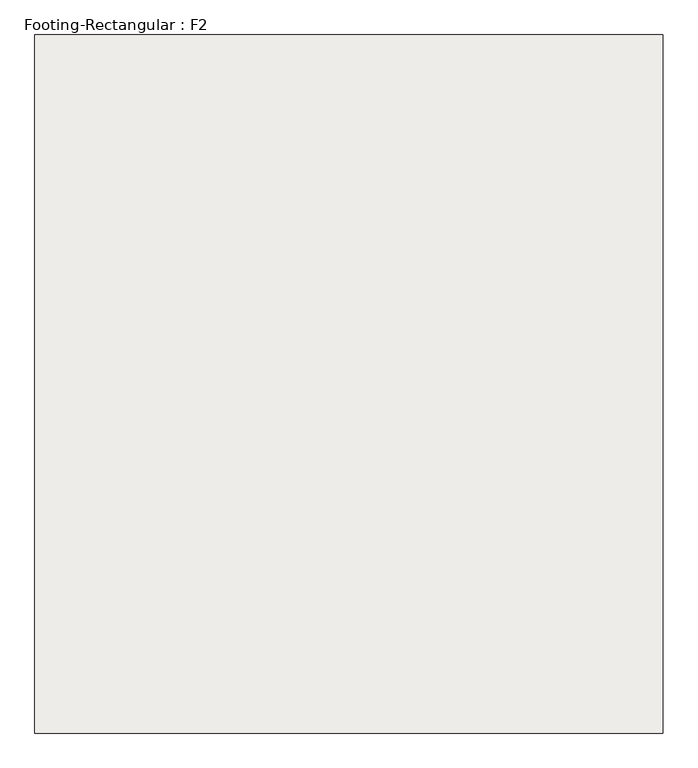
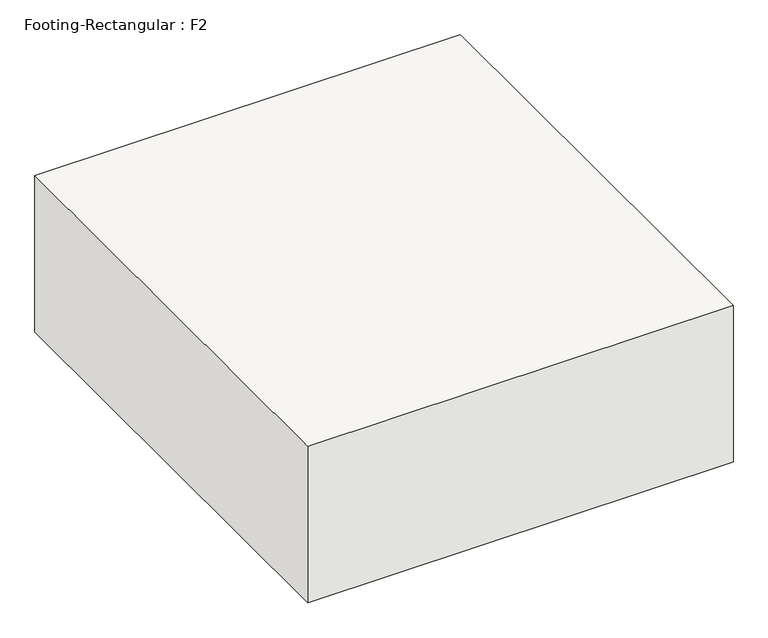
"""IFC4 building model written with IfcOpenShell, lengths in millimetres: slab geometry, Footing-Rectangular : F2."""

from ifc_helpers import new_model, si_unit, frame, origin, place, context, project, spatial, polyline, outline, extrude, source, transform, mapped, element, save


def footing_rectangular_f2_078fe2d8(model_context):
    return source(origin(), model_context, "Body", "SweptSolid", [
        extrude(outline(polyline([(685.8, 762.0), (685.8, -762.0), (-685.8, -762.0), (-685.8, 762.0), (685.8, 762.0)])), frame((0.0, 0.0, -533.4), z_axis=(0.0, 0.0, 1.0), x_axis=(1.0, 0.0, 0.0)), (0.0, 0.0, 1.0), 533.4),
    ])


if __name__ == "__main__":
    model = new_model("IFC4")
    model_context = context("Model", 3, world=origin())
    ifc_project = project(units=[si_unit("LENGTHUNIT", "METRE", prefix="MILLI")], contexts=[model_context])
    site = spatial("IfcSite", under=ifc_project)
    building = spatial("IfcBuilding", under=site)
    placement = place(None, origin())
    footing_rectangular_f2_shape = footing_rectangular_f2_078fe2d8(model_context)
    element("IfcSlab", 1, ObjectType="Footing-Rectangular : F2", at=placement, inside=building, context=model_context, shape_type="MappedRepresentation", body=[
        mapped(footing_rectangular_f2_shape, transform((0.0, 0.0, 0.0), x_axis=(1.0, 0.0, 0.0), y_axis=(0.0, 1.0, 0.0), z_axis=(0.0, 0.0, 1.0))),
    ])
    save(model, "model.ifc")

# Revit data of these elements
# Type "Footing-Rectangular : F2"
#   Width = 1371.6 mm
#   Length = 1524 mm
#   Foundation Thickness = 533.4 mm
#   Structural Material [instance default] = Concrete - Cast-in-Place Concrete
#   Assembly Code = ""
# Element 1 (IfcSlab, "Footing-Rectangular : F2")
#   Materials on its faces: "Concrete - Cast-in-Place Concrete"
# Materials
#   "Concrete - Cast-in-Place Concrete": class "Concrete", colour RGB 192 192 192, transparency 0, Cost = 0
